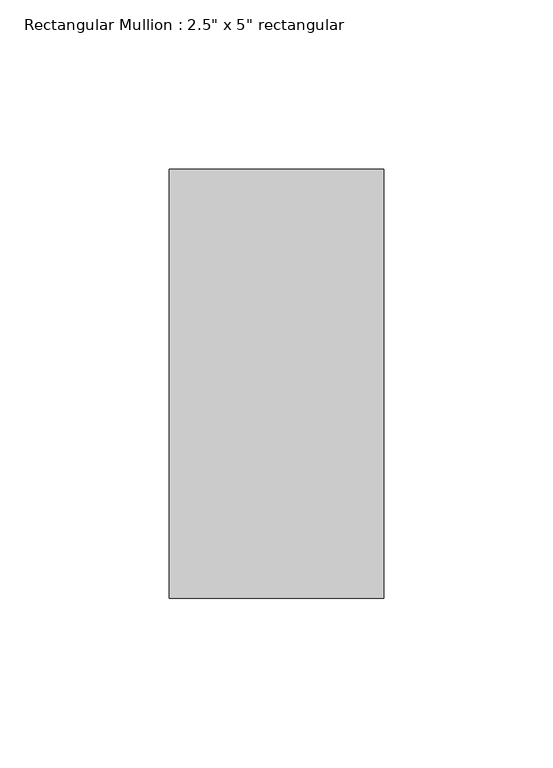
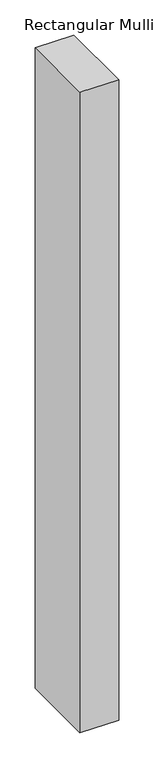
"""IFC4 building model written with IfcOpenShell, lengths in millimetres: member geometry."""

from ifc_helpers import new_model, si_unit, frame, origin, place, context, project, spatial, polyline, outline, extrude, source, transform, mapped, element, save


def member_aaf6ec4e(model_context):
    return source(origin(), model_context, "Body", "SweptSolid", [
        extrude(outline(polyline([(0.0, 63.5), (0.0, -63.5), (-63.5, -63.5), (-63.5, 63.5), (0.0, 63.5)])), frame((0.0, 0.0, -1111.25), z_axis=(0.0, 0.0, 1.0), x_axis=(1.0, 0.0, 0.0)), (0.0, 0.0, 1.0), 1111.25),
    ])


if __name__ == "__main__":
    model = new_model("IFC4")
    model_context = context("Model", 3, world=origin())
    ifc_project = project(units=[si_unit("LENGTHUNIT", "METRE", prefix="MILLI")], contexts=[model_context])
    site = spatial("IfcSite", under=ifc_project)
    building = spatial("IfcBuilding", under=site)
    placement = place(None, origin())
    member_shape = member_aaf6ec4e(model_context)
    element("IfcMember", 1, ObjectType="Rectangular Mullion : 2.5\" x 5\" rectangular", at=placement, inside=building, context=model_context, shape_type="MappedRepresentation", body=[
        mapped(member_shape, transform((0.0, 0.0, 0.0), x_axis=(1.0, 0.0, 0.0), y_axis=(0.0, 1.0, 0.0), z_axis=(0.0, 0.0, 1.0))),
    ])
    save(model, "model.ifc")

# Revit data of these elements
# Type "Rectangular Mullion : 2.5\" x 5\" rectangular"
#   built-in parameter 1007304 = 0.416667 (stored number, unit not read)
#   built-in parameter 1007301 = 0.104167 (stored number, unit not read)
#   built-in parameter 1007300 = 0.104167 (stored number, unit not read)
# Element 1 (IfcMember, "Rectangular Mullion : 2.5\" x 5\" rectangular")
#   Materials on its faces: "Aluminum"
# Materials
#   "Aluminum": class "Metal", colour RGB 247 247 247, transparency 0, Description = "Aluminum 6061", Cost = 0
